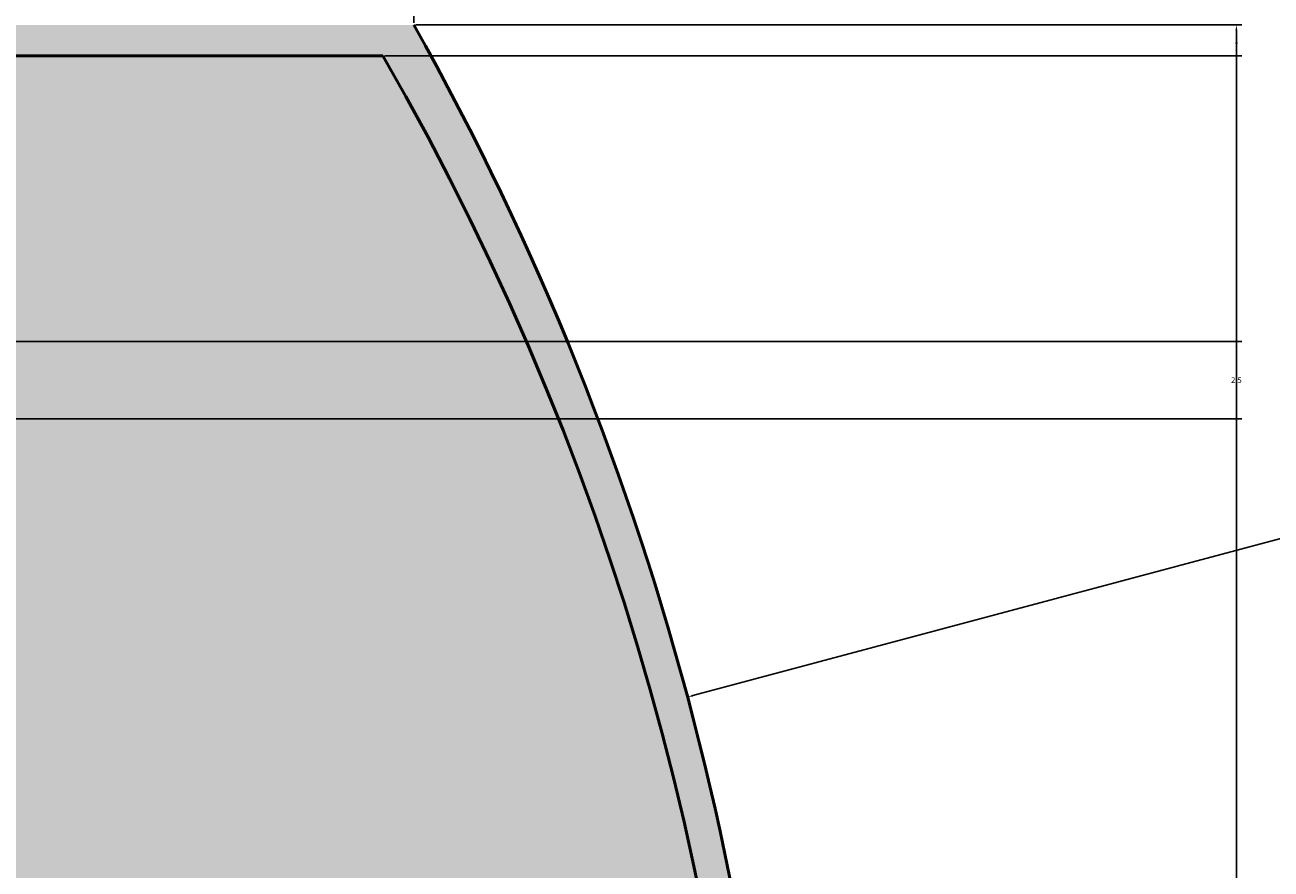
# Model space of a CAD drawing. Units: inches. Extents: x -12 to 334, y -10 to 186.
# Tile 75 of 77: x 257 to 297, y 111 to 138. Entities that reach past the tile are written whole.
import ezdxf

# ---------------------------------------------------------------- set-up
doc = ezdxf.new("R2010")
doc.units = ezdxf.units.IN
doc.header["$MEASUREMENT"] = 0
for name, color, linetype, lineweight in [('M-DIMS', 2, 'Continuous', 18), ('M-EQPM', 7, 'Continuous', 50), ('M-EQPM-PATT', 8, 'Continuous', 18)]:
    doc.layers.add(name, color=color, linetype=linetype, lineweight=lineweight)
doc.styles.get("Standard").update_dxf_attribs({"font": 'arial.ttf'})
doc.dimstyles.get("Standard").update_dxf_attribs({"dimtxt": 0.18, "dimasz": 0.18, "dimexe": 0.18, "dimexo": 0.0625, "dimgap": 0.09, "dimtad": 0, "dimtih": 1, "dimtoh": 1, "dimdec": 4, "dimzin": 0, "dimdsep": 46, "dimtxsty": 'Standard', "dimcen": 0.09, "dimadec": 0, "dimazin": 0, "dimtfac": 1, "dimtdec": 4, "dimtofl": 0, "dimtmove": 0, "dimatfit": 3, "dimfxl": 1, "dimtolj": 1, "dimtzin": 0, "dimarcsym": 0})

# ---------------------------------------------------------------- blocks, each defined once
blk = doc.blocks.new('*D5')
at = {"layer": 'Defpoints', "color": 0, "transparency": 16777216}
for p in [(58.1, 127.708), (58.1, 125.208), (295.976, 125.208)]:
    blk.add_point(p, dxfattribs=at)
at = {"layer": 'M-DIMS', "color": 0, "lineweight": -2, "transparency": 16777216}
for p, q in [((58.163, 127.708), (296.156, 127.708)), ((295.976, 127.528), (295.976, 126.64)), ((295.976, 125.388), (295.976, 126.276)), ((58.163, 125.208), (296.156, 125.208))]:
    blk.add_line(p, q, dxfattribs=at)
at = {"layer": 'M-DIMS', "color": 0, "transparency": 16777216}
for points in [[(295.946, 127.528), (296.006, 127.528), (295.976, 127.708)], [(295.946, 125.388), (296.006, 125.388), (295.976, 125.208)]]:
    blk.add_solid(points, dxfattribs=at)
at = {"layer": 'M-DIMS', "color": 0, "transparency": 16777216, "insert": (295.976, 126.458), "char_height": 0.18, "attachment_point": 5}
blk.add_mtext('\\A1;2.5', dxfattribs=at)
blk = doc.blocks.new('*D21')
at = {"layer": 'Defpoints', "color": 0, "transparency": 16777216}
for p in [(269.381, 169.385), (220.017, 154.835), (269.381, 137.943)]:
    blk.add_point(p, dxfattribs=at)
at = {"layer": 'M-DIMS', "color": 0, "lineweight": -2, "transparency": 16777216}
for p, q in [((220.017, 154.897), (220.017, 169.565)), ((220.197, 169.385), (244.301, 169.385)), ((269.201, 169.385), (245.096, 169.385)), ((269.381, 138.006), (269.381, 169.565))]:
    blk.add_line(p, q, dxfattribs=at)
at = {"layer": 'M-DIMS', "color": 0, "transparency": 16777216}
for points in [[(220.197, 169.415), (220.197, 169.355), (220.017, 169.385)], [(269.201, 169.415), (269.201, 169.355), (269.381, 169.385)]]:
    blk.add_solid(points, dxfattribs=at)
at = {"layer": 'M-DIMS', "color": 0, "transparency": 16777216, "insert": (244.699, 169.385), "char_height": 0.18, "attachment_point": 5}
blk.add_mtext('\\A1;49.36', dxfattribs=at)
blk = doc.blocks.new('*D24')
at = {"layer": 'Defpoints', "color": 0, "transparency": 16777216}
for p in [(269.381, 137.943), (269.381, 45.854), (295.976, 45.854)]:
    blk.add_point(p, dxfattribs=at)
at = {"layer": 'M-DIMS', "color": 0, "lineweight": -2, "transparency": 16777216}
for p, q in [((269.443, 137.943), (296.156, 137.943)), ((295.976, 137.763), (295.976, 92.081)), ((295.976, 46.034), (295.976, 91.717)), ((269.443, 45.854), (296.156, 45.854))]:
    blk.add_line(p, q, dxfattribs=at)
at = {"layer": 'M-DIMS', "color": 0, "transparency": 16777216}
for points in [[(295.946, 137.763), (296.006, 137.763), (295.976, 137.943)], [(295.946, 46.034), (296.006, 46.034), (295.976, 45.854)]]:
    blk.add_solid(points, dxfattribs=at)
at = {"layer": 'M-DIMS', "color": 0, "transparency": 16777216, "insert": (295.976, 91.899), "char_height": 0.18, "attachment_point": 5}
blk.add_mtext('\\A1;92.09', dxfattribs=at)
blk = doc.blocks.new('*D25')
at = {"layer": 'Defpoints', "color": 0, "transparency": 16777216}
for p in [(269.381, 137.943), (268.381, 136.943), (295.976, 136.943)]:
    blk.add_point(p, dxfattribs=at)
at = {"layer": 'M-DIMS', "color": 0, "lineweight": -2, "transparency": 16777216}
for p, q in [((269.443, 137.943), (296.156, 137.943)), ((295.976, 137.763), (295.976, 137.624)), ((295.976, 137.123), (295.976, 137.263)), ((268.443, 136.943), (296.156, 136.943))]:
    blk.add_line(p, q, dxfattribs=at)
at = {"layer": 'M-DIMS', "color": 0, "transparency": 16777216}
for points in [[(295.946, 137.763), (296.006, 137.763), (295.976, 137.943)], [(295.946, 137.123), (296.006, 137.123), (295.976, 136.943)]]:
    blk.add_solid(points, dxfattribs=at)
at = {"layer": 'M-DIMS', "color": 0, "transparency": 16777216, "insert": (295.976, 137.443), "char_height": 0.18, "attachment_point": 5}
blk.add_mtext('\\A1;1', dxfattribs=at)
blk = doc.blocks.new('*D40')
at = {"layer": 'Defpoints', "color": 0, "transparency": 16777216}
for p in [(278.229, 116.208), (187.394, 91.899)]:
    blk.add_point(p, dxfattribs=at)
at = {"layer": 'M-DIMS', "color": 0, "lineweight": -2, "transparency": 16777216}
for p, q in [((332.73, 130.793), (278.403, 116.254)), ((187.304, 91.899), (187.484, 91.899)), ((187.394, 91.809), (187.394, 91.989))]:
    blk.add_line(p, q, dxfattribs=at)
at = {"layer": 'M-DIMS', "color": 0, "transparency": 16777216}
blk.add_solid([(278.395, 116.283), (278.411, 116.225), (278.229, 116.208)], dxfattribs=at)
at = {"layer": 'M-DIMS', "color": 0, "transparency": 16777216, "insert": (333.21, 130.793), "char_height": 0.18, "attachment_point": 5}
blk.add_mtext('\\A1;R94.03', dxfattribs=at)

msp = doc.modelspace()

# ---------------------------------------------------------------- hatches: boundary and pattern name
at = {"layer": 'M-EQPM-PATT', "transparency": 33554556}
h = msp.add_hatch(color=256, dxfattribs=at)
h.set_gradient(color1=(248, 206, 179), color2=(248, 206, 179), tint=1)
h.paths.add_polyline_path([(179.7818, 136.8871), (126.9567, 136.8871), (106.1771, 100.8958), (171.5458, 100.8958)])
h.paths.add_polyline_path([(268.3808, 136.9435), (214.0166, 136.9435), (214.0166, 154.8345), (196.3421, 154.8345), (196.3421, 136.8871), (179.7818, 136.8871), (171.5458, 100.8958), (231.7758, 100.8958, -0.4142136), (251.9801, 80.6915), (279.7263, 80.6915, 0.1631825)])
at = {"layer": 'M-EQPM-PATT'}
h = msp.add_hatch(color=256, dxfattribs=at)
h.set_gradient(color1=(99, 100, 102), color2=(99, 100, 102), tint=1)
h.paths.add_polyline_path([(126.9567, 136.8871), (179.7818, 136.8871), (180.0106, 137.8871), (126.3793, 137.8871), (106.1771, 102.8958), (86.8879, 102.8958), (86.8879, 109.0583), (84.7229, 109.0583), (84.7229, 100.8958), (106.1771, 100.8958)])
h.paths.add_polyline_path([(196.3421, 152.8345), (195.3421, 152.8345), (195.3421, 137.8871), (180.0106, 137.8871), (179.7818, 136.8871), (196.3421, 136.8871)])
h.paths.add_polyline_path([(215.0166, 152.8345), (214.0166, 152.8345), (214.0166, 136.9435), (268.3808, 136.9435, -0.2673785), (268.3808, 46.8541), (249.3759, 46.8541), (249.8485, 45.8541), (269.3808, 45.8541, 0.2615891), (269.3808, 137.9435), (215.0166, 137.9435)])

# ---------------------------------------------------------------- linework, layer by layer
at = {"layer": 'M-EQPM'}
msp.add_lwpolyline([(214.0166, 154.8345), (214.0166, 136.9435), (268.3808, 136.9435)], dxfattribs=at)
for centre, radius, start, end in [((187.3936, 91.8988), 94.032, 330.681071, 29.318929), ((190.1689, 91.8988), 90.256, 330.061028, 29.938972)]:
    msp.add_arc(centre, radius, start, end, dxfattribs=at)

# ---------------------------------------------------------------- dimensions: what is measured, and where the dimension line sits
at = {"layer": 'M-DIMS'}
dim = msp.add_linear_dim(base=(269.3808, 169.3845), p1=(220.0166, 154.8345), p2=(269.3808, 137.9435), dimstyle='Standard', override={"dimdec": 2, "dimlfac": 1, "dimrnd": 0, "dimzin": 0, "dimdsep": 46, "dimlunit": 2}, dxfattribs=at)
dim.commit()
dim.dimension.update_dxf_attribs({"geometry": '*D21', "text_midpoint": (244.6987, 169.3845)})
for base, p1, p2, override, picture, middle in [((295.9756, 136.9435), (269.3808, 137.9435), (268.3808, 136.9435), {"dimdec": 0, "dimlfac": 1, "dimrnd": 0, "dimzin": 0, "dimdsep": 46, "dimlunit": 2}, '*D25', (295.9756, 137.4435)), ((295.9756, 45.8541), (269.3808, 137.9435), (269.3808, 45.8541), {"dimdec": 2, "dimlfac": 1, "dimrnd": 0, "dimzin": 0, "dimdsep": 46, "dimlunit": 2}, '*D24', (295.9756, 91.8988)), ((295.9756, 125.2078), (58.1002, 127.7078), (58.1002, 125.2078), {"dimdec": 1, "dimlfac": 1, "dimrnd": 0, "dimzin": 0, "dimdsep": 46, "dimlunit": 2}, '*D5', (295.9756, 126.4578))]:
    dim = msp.add_linear_dim(base=base, p1=p1, p2=p2, angle=90, dimstyle='Standard', override=override, dxfattribs=at)
    dim.commit()
    dim.dimension.update_dxf_attribs({"geometry": picture, "text_midpoint": middle})
dim = msp.add_radius_dim(center=(187.3936, 91.8988), mpoint=(278.2291, 116.2078), dimstyle='Standard', override={"dimdec": 2, "dimlfac": 1, "dimrnd": 0, "dimzin": 0, "dimdsep": 46, "dimlunit": 2}, dxfattribs=at)
dim.commit()
dim.dimension.update_dxf_attribs({"geometry": '*D40', "text_midpoint": (332.7304, 130.7932), "dimtype": 164})

doc.saveas('drawing.dxf')
